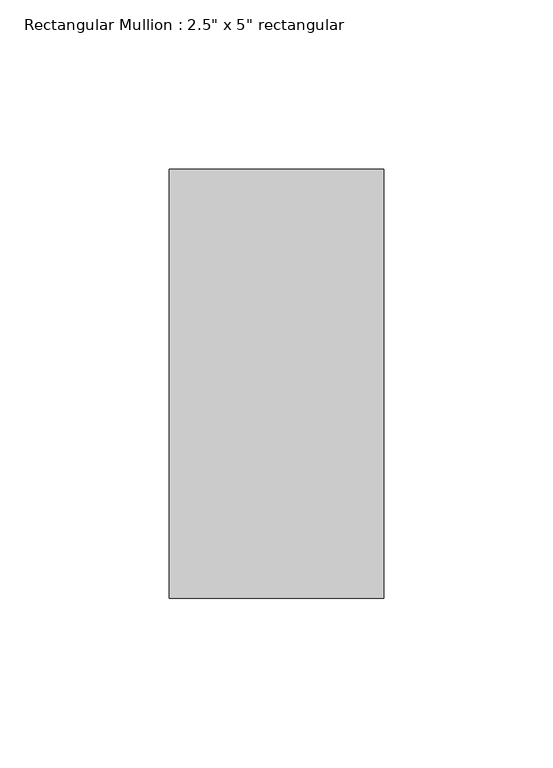
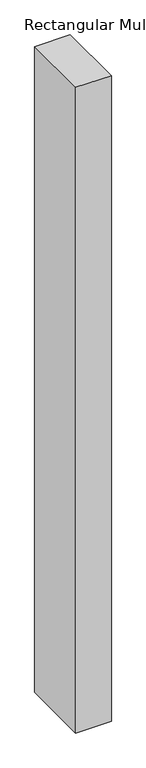
"""IFC4 building model written with IfcOpenShell, lengths in millimetres: member geometry."""

from ifc_helpers import new_model, si_unit, frame, origin, place, context, project, spatial, polyline, outline, extrude, source, transform, mapped, element, save


def member_2b49869a(model_context):
    return source(origin(), model_context, "Body", "SweptSolid", [
        extrude(outline(polyline([(31.75, 63.5), (31.75, -63.5), (-31.75, -63.5), (-31.75, 63.5), (31.75, 63.5)])), frame((0.0, 0.0, -1219.2), z_axis=(0.0, 0.0, 1.0), x_axis=(1.0, 0.0, 0.0)), (0.0, 0.0, 1.0), 1219.2),
    ])


if __name__ == "__main__":
    model = new_model("IFC4")
    model_context = context("Model", 3, world=origin())
    ifc_project = project(units=[si_unit("LENGTHUNIT", "METRE", prefix="MILLI")], contexts=[model_context])
    site = spatial("IfcSite", under=ifc_project)
    building = spatial("IfcBuilding", under=site)
    placement = place(None, origin())
    member_shape = member_2b49869a(model_context)
    element("IfcMember", 1, ObjectType="Rectangular Mullion : 2.5\" x 5\" rectangular", at=placement, inside=building, context=model_context, shape_type="MappedRepresentation", body=[
        mapped(member_shape, transform((0.0, 0.0, 0.0), x_axis=(1.0, 0.0, 0.0), y_axis=(0.0, 1.0, 0.0), z_axis=(0.0, 0.0, 1.0))),
    ])
    save(model, "model.ifc")

# Revit data of these elements
# Type "Rectangular Mullion : 2.5\" x 5\" rectangular"
#   built-in parameter 1007304 = 0.416667 (stored number, unit not read)
#   built-in parameter 1007301 = 0.104167 (stored number, unit not read)
#   built-in parameter 1007300 = 0.104167 (stored number, unit not read)
